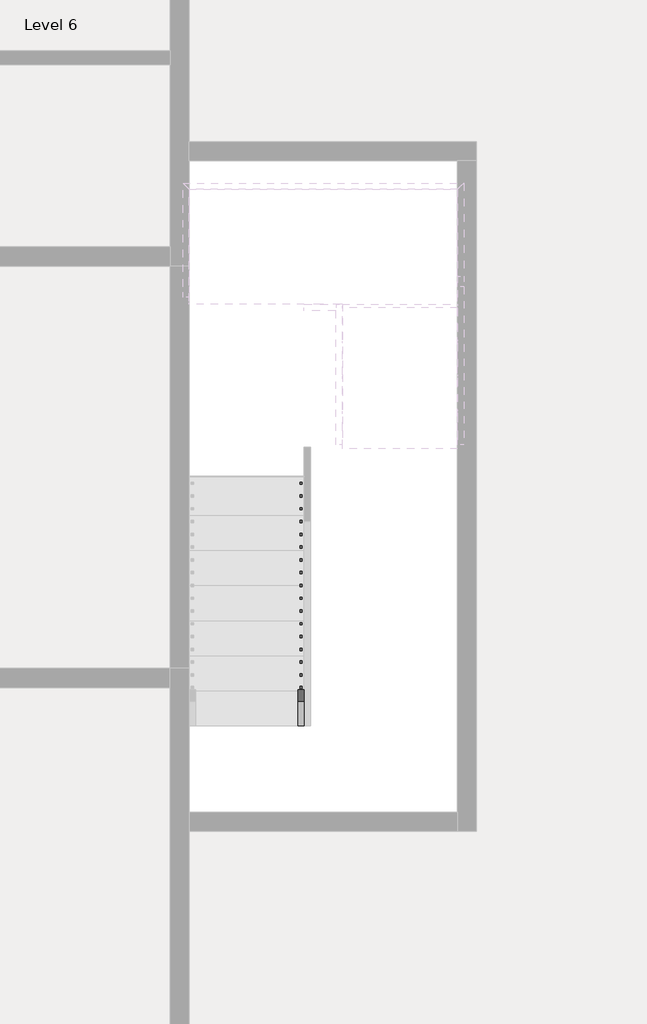
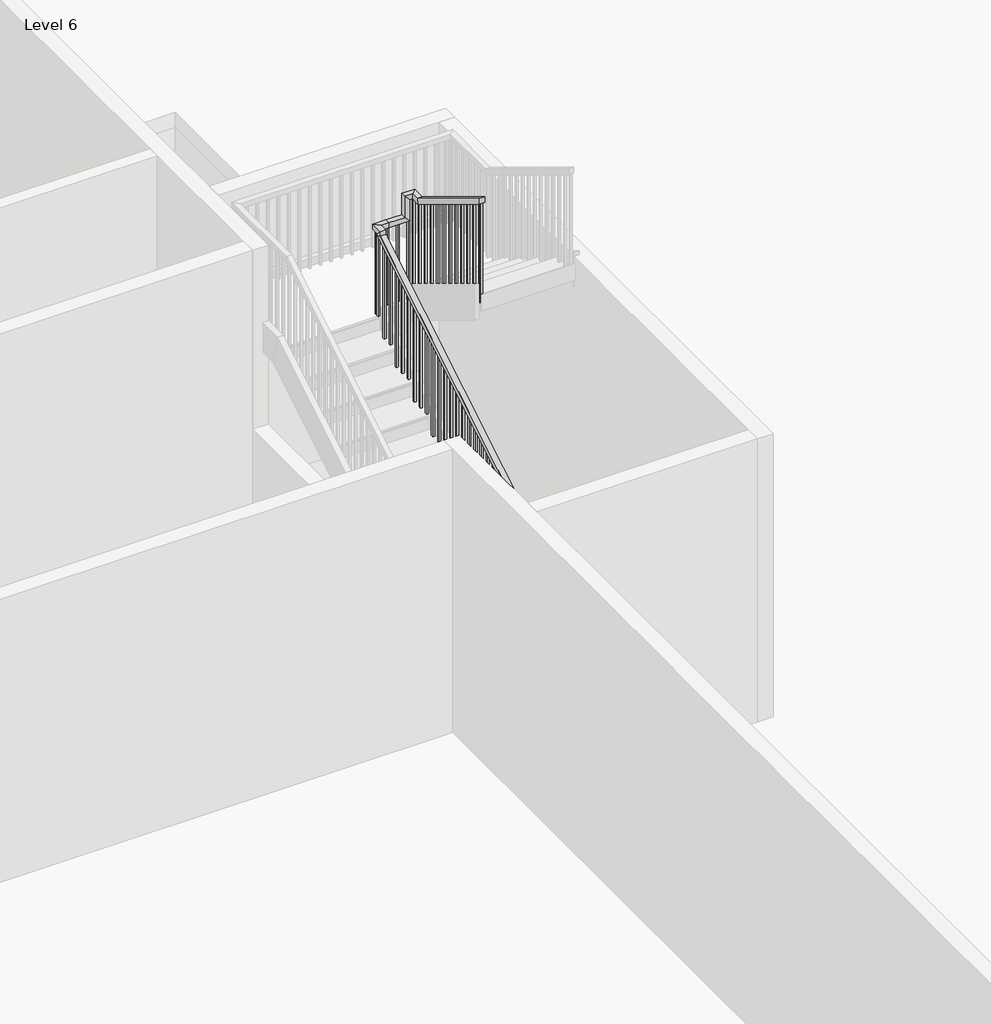
# One storey, part 7 of 8: 1 railing.
"""IFC4 building model written with IfcOpenShell, lengths in millimetres."""

from ifc_helpers import new_model, si_unit, frame, origin, place, context, project, spatial, polyline, outline, extrude, faceted_brep, element, save

model = new_model("IFC4")

# Units and contexts
model_context = context("Model", 3, world=origin())
ifc_project = project(units=[si_unit("LENGTHUNIT", "METRE", prefix="MILLI")], contexts=[model_context])

# Site, building, storey
site = spatial("IfcSite", under=ifc_project)
building = spatial("IfcBuilding", under=site)
storey = spatial("IfcBuildingStorey", under=building, Name="Level 6", Elevation=40474.6172466)

# Railing
placement = place(None, origin())
element("IfcRailing", 1, ObjectType="Handrail - Rectangular", at=placement, inside=storey, context=model_context, shape_type="SolidModel", body=[
    faceted_brep([(-2753.8415084, 19841.9216096, 41558.3505799), (-2753.8415084, 19841.9216096, 41498.9491197), (-2703.0415084, 19841.9216096, 41498.9491197), (-2703.0415084, 19841.9216096, 41558.3505799), (-2753.8415084, 23118.5216096, 43544.1687618), (-2753.8415084, 23169.3216096, 43515.5551803), (-2703.0415084, 23169.3216096, 43515.5551803), (-2703.0415084, 23118.5216096, 43544.1687618), (-2753.8415084, 23118.5216096, 43590.3505799), (-2753.8415084, 23169.3216096, 43539.5505799), (-2703.0415084, 23169.3216096, 43539.5505799), (-2703.0415084, 23118.5216096, 43590.3505799), (-2753.8415084, 23245.5216096, 43590.3505799), (-2753.8415084, 23245.5216096, 43539.5505799), (-2703.0415084, 23194.7216096, 43539.5505799), (-2703.0415084, 23194.7216096, 43590.3505799), (-2626.8415084, 23245.5216096, 43590.3505799), (-2626.8415084, 23245.5216096, 43539.5505799), (-2626.8415084, 23194.7216096, 43539.5505799), (-2626.8415084, 23194.7216096, 43590.3505799), (-2474.4415084, 23245.5216096, 43590.3505799), (-2423.6415084, 23245.5216096, 43539.5505799), (-2423.6415084, 23194.7216096, 43539.5505799), (-2474.4415084, 23194.7216096, 43590.3505799), (-2474.4415084, 23245.5216096, 43805.8657314), (-2423.6415084, 23245.5216096, 43755.0657314), (-2423.6415084, 23194.7216096, 43755.0657314), (-2474.4415084, 23194.7216096, 43805.8657314), (-2347.4415084, 23245.5216096, 43805.8657314), (-2347.4415084, 23245.5216096, 43755.0657314), (-2398.2415084, 23194.7216096, 43755.0657314), (-2398.2415084, 23194.7216096, 43805.8657314), (-2347.4415084, 23118.5216096, 43805.8657314), (-2347.4415084, 23104.3292002, 43755.0657314), (-2398.2415084, 23104.3292002, 43755.0657314), (-2398.2415084, 23118.5216096, 43805.8657314), (-2347.4415084, 22077.1216096, 44437.0172466), (-2398.2415084, 22077.1216096, 44437.0172466), (-2398.2415084, 22077.1216096, 44377.6157863), (-2347.4415084, 22077.1216096, 44377.6157863)], [[[0, 1, 2, 3]], [[1, 0, 4, 5]], [[2, 1, 5, 6]], [[3, 2, 6, 7]], [[0, 3, 7, 4]], [[5, 4, 8, 9]], [[6, 5, 9, 10]], [[7, 6, 10, 11]], [[4, 7, 11, 8]], [[9, 8, 12, 13]], [[10, 9, 13, 14]], [[11, 10, 14, 15]], [[8, 11, 15, 12]], [[13, 12, 16, 17]], [[14, 13, 17, 18]], [[15, 14, 18, 19]], [[12, 15, 19, 16]], [[17, 16, 20, 21]], [[18, 17, 21, 22]], [[19, 18, 22, 23]], [[16, 19, 23, 20]], [[21, 20, 24, 25]], [[22, 21, 25, 26]], [[23, 22, 26, 27]], [[20, 23, 27, 24]], [[25, 24, 28, 29]], [[26, 25, 29, 30]], [[27, 26, 30, 31]], [[24, 27, 31, 28]], [[29, 28, 32, 33]], [[30, 29, 33, 34]], [[31, 30, 34, 35]], [[28, 31, 35, 32]], [[36, 37, 38, 39]], [[33, 32, 36, 39]], [[34, 33, 39, 38]], [[35, 34, 38, 37]], [[32, 35, 37, 36]]]),
    extrude(outline(polyline([(22092.9966096, 44367.9945742), (22112.0466096, 44356.4491197), (22112.0466096, 43353.2839133), (22092.9966096, 43353.2839133), (22092.9966096, 44367.9945742)])), frame((-2382.3665084, 0.0, 0.0), z_axis=(1.0, 0.0, 0.0), x_axis=(0.0, 1.0, 0.0)), (0.0, 0.0, 1.0), 19.05),
    extrude(outline(polyline([(22194.5966096, 44306.4188166), (22213.6466096, 44294.8733621), (22213.6466096, 43353.2839133), (22194.5966096, 43353.2839133), (22194.5966096, 44306.4188166)])), frame((-2382.3665084, 0.0, 0.0), z_axis=(1.0, 0.0, 0.0), x_axis=(0.0, 1.0, 0.0)), (0.0, 0.0, 1.0), 19.05),
    extrude(outline(polyline([(22296.1966096, 44244.8430591), (22315.2466096, 44233.2976045), (22315.2466096, 43353.2839133), (22296.1966096, 43353.2839133), (22296.1966096, 44244.8430591)])), frame((-2382.3665084, 0.0, 0.0), z_axis=(1.0, 0.0, 0.0), x_axis=(0.0, 1.0, 0.0)), (0.0, 0.0, 1.0), 19.05),
    extrude(outline(polyline([(22397.7966096, 44183.2673015), (22416.8466096, 44171.721847), (22416.8466096, 43183.9505799), (22397.7966096, 43183.9505799), (22397.7966096, 44183.2673015)])), frame((-2382.3665084, 0.0, 0.0), z_axis=(1.0, 0.0, 0.0), x_axis=(0.0, 1.0, 0.0)), (0.0, 0.0, 1.0), 19.05),
    extrude(outline(polyline([(22499.3966096, 44121.6915439), (22518.4466096, 44110.1460894), (22518.4466096, 43183.9505799), (22499.3966096, 43183.9505799), (22499.3966096, 44121.6915439)])), frame((-2382.3665084, 0.0, 0.0), z_axis=(1.0, 0.0, 0.0), x_axis=(0.0, 1.0, 0.0)), (0.0, 0.0, 1.0), 19.05),
    extrude(outline(polyline([(22600.9966096, 44060.1157863), (22620.0466096, 44048.5703318), (22620.0466096, 43183.9505799), (22600.9966096, 43183.9505799), (22600.9966096, 44060.1157863)])), frame((-2382.3665084, 0.0, 0.0), z_axis=(1.0, 0.0, 0.0), x_axis=(0.0, 1.0, 0.0)), (0.0, 0.0, 1.0), 19.05),
    extrude(outline(polyline([(22702.5966096, 43998.5400288), (22721.6466096, 43986.9945742), (22721.6466096, 43014.6172466), (22702.5966096, 43014.6172466), (22702.5966096, 43998.5400288)])), frame((-2382.3665084, 0.0, 0.0), z_axis=(1.0, 0.0, 0.0), x_axis=(0.0, 1.0, 0.0)), (0.0, 0.0, 1.0), 19.05),
    extrude(outline(polyline([(22804.1966096, 43936.9642712), (22823.2466096, 43925.4188166), (22823.2466096, 43014.6172466), (22804.1966096, 43014.6172466), (22804.1966096, 43936.9642712)])), frame((-2382.3665084, 0.0, 0.0), z_axis=(1.0, 0.0, 0.0), x_axis=(0.0, 1.0, 0.0)), (0.0, 0.0, 1.0), 19.05),
    extrude(outline(polyline([(22905.7966096, 43875.3885136), (22924.8466096, 43863.8430591), (22924.8466096, 43014.6172466), (22905.7966096, 43014.6172466), (22905.7966096, 43875.3885136)])), frame((-2382.3665084, 0.0, 0.0), z_axis=(1.0, 0.0, 0.0), x_axis=(0.0, 1.0, 0.0)), (0.0, 0.0, 1.0), 19.05),
    extrude(outline(polyline([(23007.3966096, 43813.812756), (23026.4466096, 43802.2673015), (23026.4466096, 42845.2839133), (23007.3966096, 42845.2839133), (23007.3966096, 43813.812756)])), frame((-2382.3665084, 0.0, 0.0), z_axis=(1.0, 0.0, 0.0), x_axis=(0.0, 1.0, 0.0)), (0.0, 0.0, 1.0), 19.05),
    extrude(outline(polyline([(23108.9966096, 43752.2369985), (23128.0466096, 43740.6915439), (23128.0466096, 42845.2839133), (23108.9966096, 42845.2839133), (23108.9966096, 43752.2369985)])), frame((-2382.3665084, 0.0, 0.0), z_axis=(1.0, 0.0, 0.0), x_axis=(0.0, 1.0, 0.0)), (0.0, 0.0, 1.0), 19.05),
    extrude(outline(polyline([(-2433.1665084, 23210.5966096), (-2433.1665084, 23229.6466096), (-2414.1165084, 23229.6466096), (-2414.1165084, 23210.5966096), (-2433.1665084, 23210.5966096)])), frame((0.0, 0.0, 42675.9505799), z_axis=(0.0, 0.0, 1.0), x_axis=(1.0, 0.0, 0.0)), (0.0, 0.0, 1.0), 1079.1151515),
    extrude(outline(polyline([(-2534.7665084, 23210.5966096), (-2534.7665084, 23229.6466096), (-2515.7165084, 23229.6466096), (-2515.7165084, 23210.5966096), (-2534.7665084, 23210.5966096)])), frame((0.0, 0.0, 42675.9505799), z_axis=(0.0, 0.0, 1.0), x_axis=(1.0, 0.0, 0.0)), (0.0, 0.0, 1.0), 863.6),
    extrude(outline(polyline([(-2636.3665084, 23210.5966096), (-2636.3665084, 23229.6466096), (-2617.3165084, 23229.6466096), (-2617.3165084, 23210.5966096), (-2636.3665084, 23210.5966096)])), frame((0.0, 0.0, 42675.9505799), z_axis=(0.0, 0.0, 1.0), x_axis=(1.0, 0.0, 0.0)), (0.0, 0.0, 1.0), 863.6),
    extrude(outline(polyline([(-2718.9165084, 23185.1966096), (-2737.9665084, 23185.1966096), (-2737.9665084, 23204.2466096), (-2718.9165084, 23204.2466096), (-2718.9165084, 23185.1966096)])), frame((0.0, 0.0, 42675.9505799), z_axis=(0.0, 0.0, 1.0), x_axis=(1.0, 0.0, 0.0)), (0.0, 0.0, 1.0), 863.6),
    extrude(outline(polyline([(23083.5966096, 43463.6006348), (23102.6466096, 43475.1460894), (23102.6466096, 42506.6172466), (23083.5966096, 42506.6172466), (23083.5966096, 43463.6006348)])), frame((-2737.9665084, 0.0, 0.0), z_axis=(1.0, 0.0, 0.0), x_axis=(0.0, 1.0, 0.0)), (0.0, 0.0, 1.0), 19.05),
    extrude(outline(polyline([(22981.9966096, 43402.0248773), (23001.0466096, 43413.5703318), (23001.0466096, 42506.6172466), (22981.9966096, 42506.6172466), (22981.9966096, 43402.0248773)])), frame((-2737.9665084, 0.0, 0.0), z_axis=(1.0, 0.0, 0.0), x_axis=(0.0, 1.0, 0.0)), (0.0, 0.0, 1.0), 19.05),
    extrude(outline(polyline([(22880.3966096, 43340.4491197), (22899.4466096, 43351.9945742), (22899.4466096, 42337.2839133), (22880.3966096, 42337.2839133), (22880.3966096, 43340.4491197)])), frame((-2737.9665084, 0.0, 0.0), z_axis=(1.0, 0.0, 0.0), x_axis=(0.0, 1.0, 0.0)), (0.0, 0.0, 1.0), 19.05),
    extrude(outline(polyline([(22778.7966096, 43278.8733621), (22797.8466096, 43290.4188166), (22797.8466096, 42337.2839133), (22778.7966096, 42337.2839133), (22778.7966096, 43278.8733621)])), frame((-2737.9665084, 0.0, 0.0), z_axis=(1.0, 0.0, 0.0), x_axis=(0.0, 1.0, 0.0)), (0.0, 0.0, 1.0), 19.05),
    extrude(outline(polyline([(22677.1966096, 43217.2976045), (22696.2466096, 43228.8430591), (22696.2466096, 42337.2839133), (22677.1966096, 42337.2839133), (22677.1966096, 43217.2976045)])), frame((-2737.9665084, 0.0, 0.0), z_axis=(1.0, 0.0, 0.0), x_axis=(0.0, 1.0, 0.0)), (0.0, 0.0, 1.0), 19.05),
    extrude(outline(polyline([(22575.5966096, 43155.721847), (22594.6466096, 43167.2673015), (22594.6466096, 42167.9505799), (22575.5966096, 42167.9505799), (22575.5966096, 43155.721847)])), frame((-2737.9665084, 0.0, 0.0), z_axis=(1.0, 0.0, 0.0), x_axis=(0.0, 1.0, 0.0)), (0.0, 0.0, 1.0), 19.05),
    extrude(outline(polyline([(22473.9966096, 43094.1460894), (22493.0466096, 43105.6915439), (22493.0466096, 42167.9505799), (22473.9966096, 42167.9505799), (22473.9966096, 43094.1460894)])), frame((-2737.9665084, 0.0, 0.0), z_axis=(1.0, 0.0, 0.0), x_axis=(0.0, 1.0, 0.0)), (0.0, 0.0, 1.0), 19.05),
    extrude(outline(polyline([(22372.3966096, 43032.5703318), (22391.4466096, 43044.1157863), (22391.4466096, 42167.9505799), (22372.3966096, 42167.9505799), (22372.3966096, 43032.5703318)])), frame((-2737.9665084, 0.0, 0.0), z_axis=(1.0, 0.0, 0.0), x_axis=(0.0, 1.0, 0.0)), (0.0, 0.0, 1.0), 19.05),
    extrude(outline(polyline([(22270.7966096, 42970.9945742), (22289.8466096, 42982.5400288), (22289.8466096, 41998.6172466), (22270.7966096, 41998.6172466), (22270.7966096, 42970.9945742)])), frame((-2737.9665084, 0.0, 0.0), z_axis=(1.0, 0.0, 0.0), x_axis=(0.0, 1.0, 0.0)), (0.0, 0.0, 1.0), 19.05),
    extrude(outline(polyline([(22169.1966096, 42909.4188166), (22188.2466096, 42920.9642712), (22188.2466096, 41998.6172466), (22169.1966096, 41998.6172466), (22169.1966096, 42909.4188166)])), frame((-2737.9665084, 0.0, 0.0), z_axis=(1.0, 0.0, 0.0), x_axis=(0.0, 1.0, 0.0)), (0.0, 0.0, 1.0), 19.05),
    extrude(outline(polyline([(22067.5966096, 42847.8430591), (22086.6466096, 42859.3885136), (22086.6466096, 41998.6172466), (22067.5966096, 41998.6172466), (22067.5966096, 42847.8430591)])), frame((-2737.9665084, 0.0, 0.0), z_axis=(1.0, 0.0, 0.0), x_axis=(0.0, 1.0, 0.0)), (0.0, 0.0, 1.0), 19.05),
    extrude(outline(polyline([(21965.9966096, 42786.2673015), (21985.0466096, 42797.812756), (21985.0466096, 41829.2839133), (21965.9966096, 41829.2839133), (21965.9966096, 42786.2673015)])), frame((-2737.9665084, 0.0, 0.0), z_axis=(1.0, 0.0, 0.0), x_axis=(0.0, 1.0, 0.0)), (0.0, 0.0, 1.0), 19.05),
    extrude(outline(polyline([(21864.3966096, 42724.6915439), (21883.4466096, 42736.2369985), (21883.4466096, 41829.2839133), (21864.3966096, 41829.2839133), (21864.3966096, 42724.6915439)])), frame((-2737.9665084, 0.0, 0.0), z_axis=(1.0, 0.0, 0.0), x_axis=(0.0, 1.0, 0.0)), (0.0, 0.0, 1.0), 19.05),
    extrude(outline(polyline([(21762.7966096, 42663.1157863), (21781.8466096, 42674.6612409), (21781.8466096, 41659.9505799), (21762.7966096, 41659.9505799), (21762.7966096, 42663.1157863)])), frame((-2737.9665084, 0.0, 0.0), z_axis=(1.0, 0.0, 0.0), x_axis=(0.0, 1.0, 0.0)), (0.0, 0.0, 1.0), 19.05),
    extrude(outline(polyline([(21661.1966096, 42601.5400288), (21680.2466096, 42613.0854833), (21680.2466096, 41659.9505799), (21661.1966096, 41659.9505799), (21661.1966096, 42601.5400288)])), frame((-2737.9665084, 0.0, 0.0), z_axis=(1.0, 0.0, 0.0), x_axis=(0.0, 1.0, 0.0)), (0.0, 0.0, 1.0), 19.05),
    extrude(outline(polyline([(21559.5966096, 42539.9642712), (21578.6466096, 42551.5097257), (21578.6466096, 41659.9505799), (21559.5966096, 41659.9505799), (21559.5966096, 42539.9642712)])), frame((-2737.9665084, 0.0, 0.0), z_axis=(1.0, 0.0, 0.0), x_axis=(0.0, 1.0, 0.0)), (0.0, 0.0, 1.0), 19.05),
    extrude(outline(polyline([(21457.9966096, 42478.3885136), (21477.0466096, 42489.9339682), (21477.0466096, 41490.6172466), (21457.9966096, 41490.6172466), (21457.9966096, 42478.3885136)])), frame((-2737.9665084, 0.0, 0.0), z_axis=(1.0, 0.0, 0.0), x_axis=(0.0, 1.0, 0.0)), (0.0, 0.0, 1.0), 19.05),
    extrude(outline(polyline([(21356.3966096, 42416.812756), (21375.4466096, 42428.3582106), (21375.4466096, 41490.6172466), (21356.3966096, 41490.6172466), (21356.3966096, 42416.812756)])), frame((-2737.9665084, 0.0, 0.0), z_axis=(1.0, 0.0, 0.0), x_axis=(0.0, 1.0, 0.0)), (0.0, 0.0, 1.0), 19.05),
    extrude(outline(polyline([(21254.7966096, 42355.2369985), (21273.8466096, 42366.782453), (21273.8466096, 41490.6172466), (21254.7966096, 41490.6172466), (21254.7966096, 42355.2369985)])), frame((-2737.9665084, 0.0, 0.0), z_axis=(1.0, 0.0, 0.0), x_axis=(0.0, 1.0, 0.0)), (0.0, 0.0, 1.0), 19.05),
    extrude(outline(polyline([(21153.1966096, 42293.6612409), (21172.2466096, 42305.2066954), (21172.2466096, 41321.2839133), (21153.1966096, 41321.2839133), (21153.1966096, 42293.6612409)])), frame((-2737.9665084, 0.0, 0.0), z_axis=(1.0, 0.0, 0.0), x_axis=(0.0, 1.0, 0.0)), (0.0, 0.0, 1.0), 19.05),
    extrude(outline(polyline([(21051.5966096, 42232.0854833), (21070.6466096, 42243.6309379), (21070.6466096, 41321.2839133), (21051.5966096, 41321.2839133), (21051.5966096, 42232.0854833)])), frame((-2737.9665084, 0.0, 0.0), z_axis=(1.0, 0.0, 0.0), x_axis=(0.0, 1.0, 0.0)), (0.0, 0.0, 1.0), 19.05),
    extrude(outline(polyline([(20949.9966096, 42170.5097257), (20969.0466096, 42182.0551803), (20969.0466096, 41321.2839133), (20949.9966096, 41321.2839133), (20949.9966096, 42170.5097257)])), frame((-2737.9665084, 0.0, 0.0), z_axis=(1.0, 0.0, 0.0), x_axis=(0.0, 1.0, 0.0)), (0.0, 0.0, 1.0), 19.05),
    extrude(outline(polyline([(20848.3966096, 42108.9339682), (20867.4466096, 42120.4794227), (20867.4466096, 41151.9505799), (20848.3966096, 41151.9505799), (20848.3966096, 42108.9339682)])), frame((-2737.9665084, 0.0, 0.0), z_axis=(1.0, 0.0, 0.0), x_axis=(0.0, 1.0, 0.0)), (0.0, 0.0, 1.0), 19.05),
    extrude(outline(polyline([(20746.7966096, 42047.3582106), (20765.8466096, 42058.9036651), (20765.8466096, 41151.9505799), (20746.7966096, 41151.9505799), (20746.7966096, 42047.3582106)])), frame((-2737.9665084, 0.0, 0.0), z_axis=(1.0, 0.0, 0.0), x_axis=(0.0, 1.0, 0.0)), (0.0, 0.0, 1.0), 19.05),
    extrude(outline(polyline([(20645.1966096, 41985.782453), (20664.2466096, 41997.3279076), (20664.2466096, 40982.6172466), (20645.1966096, 40982.6172466), (20645.1966096, 41985.782453)])), frame((-2737.9665084, 0.0, 0.0), z_axis=(1.0, 0.0, 0.0), x_axis=(0.0, 1.0, 0.0)), (0.0, 0.0, 1.0), 19.05),
    extrude(outline(polyline([(20543.5966096, 41924.2066954), (20562.6466096, 41935.75215), (20562.6466096, 40982.6172466), (20543.5966096, 40982.6172466), (20543.5966096, 41924.2066954)])), frame((-2737.9665084, 0.0, 0.0), z_axis=(1.0, 0.0, 0.0), x_axis=(0.0, 1.0, 0.0)), (0.0, 0.0, 1.0), 19.05),
    extrude(outline(polyline([(20441.9966096, 41862.6309379), (20461.0466096, 41874.1763924), (20461.0466096, 40982.6172466), (20441.9966096, 40982.6172466), (20441.9966096, 41862.6309379)])), frame((-2737.9665084, 0.0, 0.0), z_axis=(1.0, 0.0, 0.0), x_axis=(0.0, 1.0, 0.0)), (0.0, 0.0, 1.0), 19.05),
    extrude(outline(polyline([(20340.3966096, 41801.0551803), (20359.4466096, 41812.6006348), (20359.4466096, 40813.2839133), (20340.3966096, 40813.2839133), (20340.3966096, 41801.0551803)])), frame((-2737.9665084, 0.0, 0.0), z_axis=(1.0, 0.0, 0.0), x_axis=(0.0, 1.0, 0.0)), (0.0, 0.0, 1.0), 19.05),
    extrude(outline(polyline([(20238.7966096, 41739.4794227), (20257.8466096, 41751.0248773), (20257.8466096, 40813.2839133), (20238.7966096, 40813.2839133), (20238.7966096, 41739.4794227)])), frame((-2737.9665084, 0.0, 0.0), z_axis=(1.0, 0.0, 0.0), x_axis=(0.0, 1.0, 0.0)), (0.0, 0.0, 1.0), 19.05),
    extrude(outline(polyline([(20137.1966096, 41677.9036651), (20156.2466096, 41689.4491197), (20156.2466096, 40813.2839133), (20137.1966096, 40813.2839133), (20137.1966096, 41677.9036651)])), frame((-2737.9665084, 0.0, 0.0), z_axis=(1.0, 0.0, 0.0), x_axis=(0.0, 1.0, 0.0)), (0.0, 0.0, 1.0), 19.05),
    extrude(outline(polyline([(20035.5966096, 41616.3279076), (20054.6466096, 41627.8733621), (20054.6466096, 40643.9505799), (20035.5966096, 40643.9505799), (20035.5966096, 41616.3279076)])), frame((-2737.9665084, 0.0, 0.0), z_axis=(1.0, 0.0, 0.0), x_axis=(0.0, 1.0, 0.0)), (0.0, 0.0, 1.0), 19.05),
    extrude(outline(polyline([(19933.9966096, 41554.75215), (19953.0466096, 41566.2976045), (19953.0466096, 40643.9505799), (19933.9966096, 40643.9505799), (19933.9966096, 41554.75215)])), frame((-2737.9665084, 0.0, 0.0), z_axis=(1.0, 0.0, 0.0), x_axis=(0.0, 1.0, 0.0)), (0.0, 0.0, 1.0), 19.05),
    extrude(outline(polyline([(-2382.3665084, 23210.5966096), (-2382.3665084, 23229.6466096), (-2363.3165084, 23229.6466096), (-2363.3165084, 23210.5966096), (-2382.3665084, 23210.5966096)])), frame((0.0, 0.0, 42675.9505799), z_axis=(0.0, 0.0, 1.0), x_axis=(1.0, 0.0, 0.0)), (0.0, 0.0, 1.0), 1079.1151515),
    extrude(outline(polyline([(-2718.9165084, 23210.5966096), (-2737.9665084, 23210.5966096), (-2737.9665084, 23229.6466096), (-2718.9165084, 23229.6466096), (-2718.9165084, 23210.5966096)])), frame((0.0, 0.0, 42675.9505799), z_axis=(0.0, 0.0, 1.0), x_axis=(1.0, 0.0, 0.0)), (0.0, 0.0, 1.0), 863.6),
    extrude(outline(polyline([(22077.1216096, 44377.6157863), (22096.1716096, 44366.0703318), (22096.1716096, 43353.2839133), (22077.1216096, 43353.2839133), (22077.1216096, 44377.6157863)])), frame((-2382.3665084, 0.0, 0.0), z_axis=(1.0, 0.0, 0.0), x_axis=(0.0, 1.0, 0.0)), (0.0, 0.0, 1.0), 19.05),
    extrude(outline(polyline([(19841.9216096, 41498.9491197), (19860.9716096, 41510.4945742), (19860.9716096, 40643.9505799), (19841.9216096, 40643.9505799), (19841.9216096, 41498.9491197)])), frame((-2737.9665084, 0.0, 0.0), z_axis=(1.0, 0.0, 0.0), x_axis=(0.0, 1.0, 0.0)), (0.0, 0.0, 1.0), 19.05),
])

save(model, "model.ifc")

# Revit data of these elements
# Type "Handrail - Rectangular"
#   Assembly Code = "C2010400"
#   built-in parameter 1008612 = 0.0416667 (stored number, unit not read)
#   built-in parameter 1008611 = 0.0416667 (stored number, unit not read)
#   built-in parameter 1008609 = 0.333333 (stored number, unit not read)
#   built-in parameter 1008604 = 0.166667 (stored number, unit not read)
#   built-in parameter 1008603 = 0.166667 (stored number, unit not read)
#   Railing Height = 3' - 0"
#   built-in parameter 1008630 = 2
#   built-in parameter 1008610 = 2
#   built-in parameter 1008618 = Baluster - Square : 3/4"
# Element 1 (IfcRailing, "Handrail - Rectangular")
#   Phase Created = New Construction
